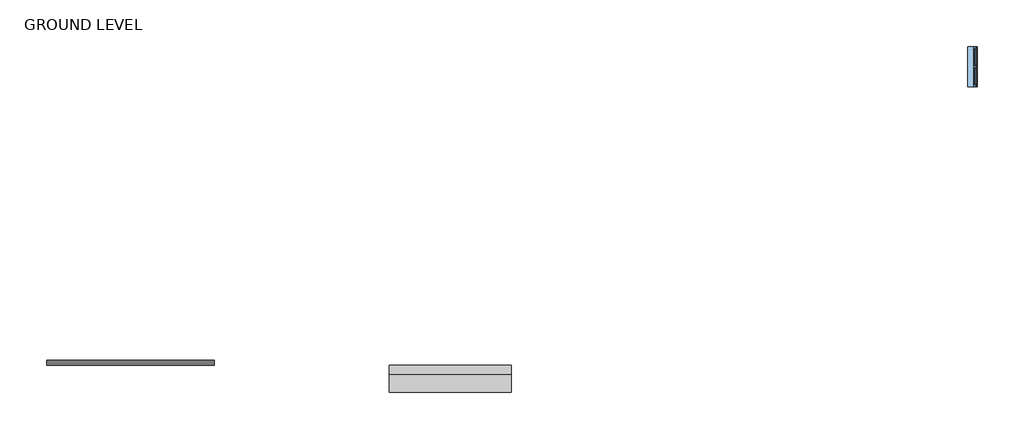
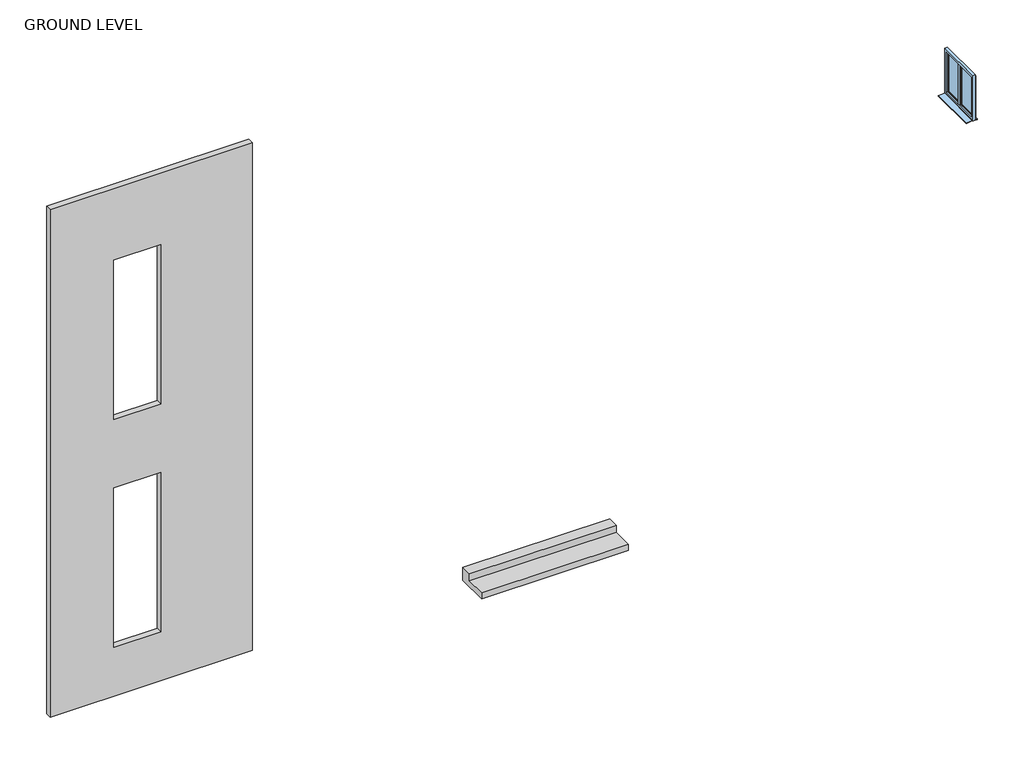
# One storey: 2 proxies, 1 window.
"""IFC4 building model written with IfcOpenShell, lengths in millimetres."""

from ifc_helpers import new_model, si_unit, origin, place, context, project, spatial, transform, mapped, element, save
from components import generic_models_1_generic_models_1_a9dcc39e, generic_models_33_generic_models_33_1b0ebd61, w2_0001_4_x_4_window_9dec5fc7

model = new_model("IFC4")

# Units and contexts
model_context = context("Model", 3, world=origin())
ifc_project = project(units=[si_unit("LENGTHUNIT", "METRE", prefix="MILLI")], contexts=[model_context])

# Site, building, storey
site = spatial("IfcSite", under=ifc_project)
building = spatial("IfcBuilding", under=site)
storey = spatial("IfcBuildingStorey", under=building, Name="GROUND LEVEL", Elevation=0.0)

# Proxies
placement = place(None, origin())
generic_models_1_generic_models_1_shape = generic_models_1_generic_models_1_a9dcc39e(model_context)
element("IfcBuildingElementProxy", 1, Name="Generic Models 1 : Generic Models 1", ObjectType="Generic Models 1 : Generic Models 1", at=placement, inside=storey, context=model_context, shape_type="MappedRepresentation", body=[
    mapped(generic_models_1_generic_models_1_shape, transform((0.0, 0.0, 0.0), x_axis=(1.0, 0.0, 0.0), y_axis=(0.0, 1.0, 0.0), z_axis=(0.0, 0.0, 1.0))),
])
generic_models_33_generic_models_33_shape = generic_models_33_generic_models_33_1b0ebd61(model_context)
element("IfcBuildingElementProxy", 2, Name="Generic Models 33 : Generic Models 33", ObjectType="Generic Models 33 : Generic Models 33", at=placement, inside=storey, context=model_context, shape_type="MappedRepresentation", body=[
    mapped(generic_models_33_generic_models_33_shape, transform((0.0, 0.0, 0.0), x_axis=(1.0, 0.0, 0.0), y_axis=(0.0, 1.0, 0.0), z_axis=(0.0, 0.0, 1.0))),
])

# Window
w2_0001_4_x_4_window_shape = w2_0001_4_x_4_window_9dec5fc7(model_context)
element("IfcWindow", 3, ObjectType="w2.0001 : 4' X 4' WINDOW", at=placement, inside=storey, context=model_context, shape_type="MappedRepresentation", body=[
    mapped(w2_0001_4_x_4_window_shape, transform((12927.3128058, -2167.3794704, -85.6), x_axis=(0.0, 1.0, 0.0), y_axis=(-1.0, 0.0, 0.0), z_axis=(0.0, 0.0, 1.0))),
])

save(model, "model.ifc")

# Revit data of these elements
# Type "w2.0001 : 4' X 4' WINDOW"
#   Type Mark = "21"
#   Operation = "DoublePanelVertical"
#   Keynote = "16.05.01"
#   Analytic Construction = "<None>"
#   Rough Width = 4' - 0"
#   Rough Height = 4' - 0"
#   Rahmentiefe = 0' - 2.3622"
#   Rahmenhöhe unten = 0' - 3.14961"
#   Rahmehöhe oben = 0' - 3.14961"
#   Rahmenbreite = 0' - 2.3622"
#   Height = 4' - 0"
#   Flügeltiefe = 0' - 2.3622"
#   Flügelbreite = 0' - 2.3622"
#   Einbautiefe (von außen) [instance default] = 0' - 5.51181"
#   Width = 4' - 0"
#   Kippflügel [instance default] = yes
#   Drehflügel im Grundriß darstellen [instance default] = no
#   Drehflügel [instance default] = yes
#   Define Thermal Properties by = 1
#   Rahmen [instance default] = none
#   Glas [instance default] = none
#   Flügel [instance default] = none
#   Fensterbank aussen [instance default] = none
#   Fensterbank innen [instance default] = none
#   Wall Closure = (empty or 0)
# Element 1 (IfcBuildingElementProxy, "Generic Models 1 : Generic Models 1")
#   Phase Created = New Construction
#   Materials on its faces: "WALL ACCENT 6\""
# Element 2 (IfcBuildingElementProxy, "Generic Models 33 : Generic Models 33")
#   Phase Created = New Construction
#   Materials on its faces: "Tile, Porcelain, 4in"
# Element 3 (IfcWindow, "w2.0001 : 4' X 4' WINDOW")
#   Mark = "102"
#   Einbautiefe (von außen) = 0' - 5.51181"
#   Kippflügel = yes
#   Drehflügel im Grundriß darstellen = no
#   Drehflügel = yes
#   Rahmen = none
#   Glas = none
#   Flügel = none
#   Fensterbank innen = none
#   Fensterbank aussen = none
#   Phase Created = New Construction
#   Materials on its faces: "Fenster - Kunststoff", "Fenster - Kunststoff weiss", "Glass", "Fenster - Holz"
# Materials
#   "WALL ACCENT 6\"": class "Generic", colour RGB 120 120 120, transparency 0, Cost = 0
#   "Tile, Porcelain, 4in": class "Generic", colour RGB 89 87 158, transparency 0, Description = "Porcelain tile, 4\", white", Cost = 0
#   "Fenster - Kunststoff": colour RGB 249 249 249, transparency 0
#   "Fenster - Kunststoff weiss": colour RGB 249 249 249, transparency 0
#   "Glass": class "Glass", colour RGB 0 128 192, transparency 0.75, Description = "Soda Lime Glass", Cost = 0
#   "Fenster - Holz": colour RGB 216 135 75, transparency 0
